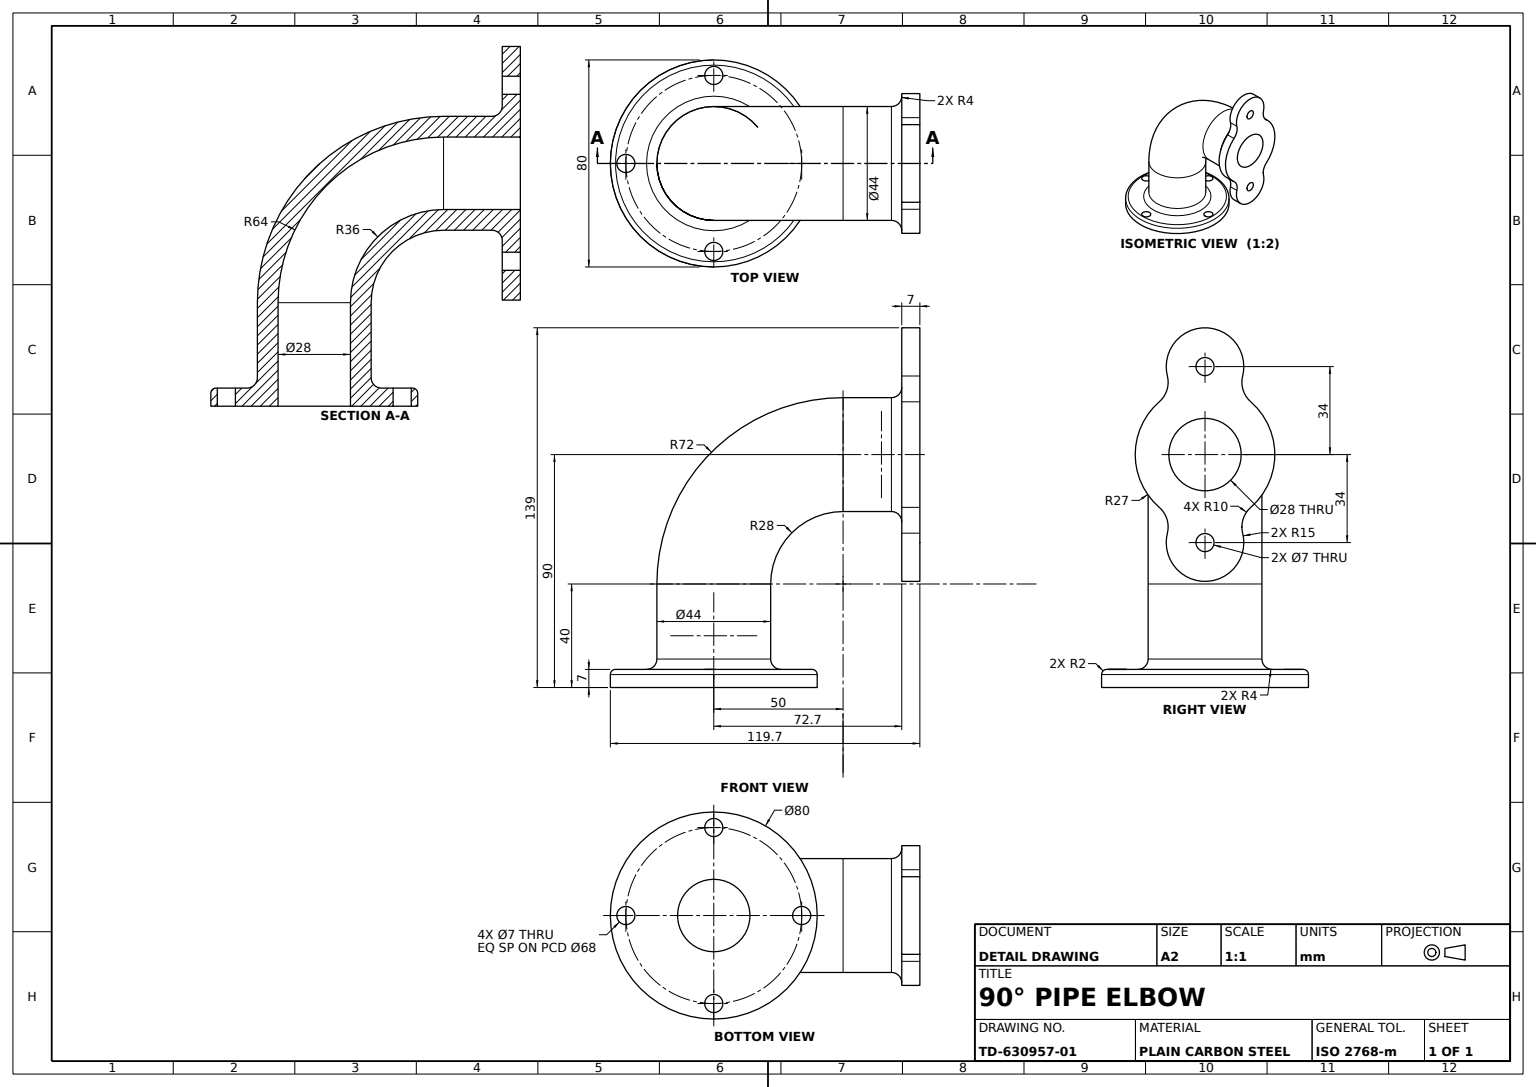
from build123d import *

# Parameters (mm, degrees)
OVAL_FLANGE_SKETCH_R               = 14
OVAL_FLANGE_SKETCH_R_2             = 3.5
OVAL_FLANGE_DEPTH                  = 3.5
PIPE_SECTION_SKETCH_44X_28_R       = 22
PIPE_SECTION_SKETCH_44X_28_R_2     = 14
ROUND_START                        = 7
ROUND_FLANGE_SKETCH_R              = 40
ROUND_FLANGE_SKETCH_R_2            = 14
ROUND_FLANGE_80_DEPTH              = 7
PIPE_TO_FLANGE_FILLETS_R4_R        = 4
ROUND_FLANGE_EDGE_FILLET_R2_R      = 2
ROUND_FLANGE_BOLT_HOLES_SKETCH_R   = 3.5
ROUND_FLANGE_BOLT_HOLES_4X_7_DEPTH = 10


with BuildPart() as part:
    # Oval Flange Sketch → Oval Flange (new, symmetric)
    with BuildSketch(Plane(origin=(0, 0, 0), x_dir=(0, 0, -1), z_dir=(1, 0, 0))):
        with BuildLine():
            ThreePointArc((17.699378464, -20.389507154), (27, 0), (17.699378464, 20.389507154))
            ThreePointArc((17.699378464, 20.389507154), (14.717914983, 24.932911413), (14.552822293, 30.364705882))
            ThreePointArc((14.552822293, 30.364705882), (0, 49), (-14.552822293, 30.364705882))
            ThreePointArc((-14.552822293, 30.364705882), (-14.717914983, 24.932911413), (-17.699378464, 20.389507154))
            ThreePointArc((-17.699378464, 20.389507154), (-27, 0), (-17.699378464, -20.389507154))
            ThreePointArc((-17.699378464, -20.389507154), (-14.717914983, -24.932911413), (-14.552822293, -30.364705882))
            ThreePointArc((-14.552822293, -30.364705882), (0, -49), (14.552822293, -30.364705882))
            ThreePointArc((14.552822293, -30.364705882), (14.717914983, -24.932911413), (17.699378464, -20.389507154))
        make_face()
        Circle(OVAL_FLANGE_SKETCH_R, mode=Mode.SUBTRACT)
        with Locations((0, 34)):
            Circle(OVAL_FLANGE_SKETCH_R_2, mode=Mode.SUBTRACT)
        with Locations((0, -34)):
            Circle(OVAL_FLANGE_SKETCH_R_2, mode=Mode.SUBTRACT)
    extrude(amount=OVAL_FLANGE_DEPTH, both=True)

    # Pipe Elbow Sweep: sweep along a path in Elbow Path Sketch
    with BuildLine(Plane.XY) as pipe_elbow_sweep_path:
        Line((0, 0), (-26.195643288, 0))
        ThreePointArc((-26.195643288, 0), (-61.550982347, -14.644660941), (-76.195643288, -50))
        Line((-76.195643288, -50), (-76.195643288, -83))
    # Pipe Section Sketch Ø44xØ28 → Pipe Elbow Sweep (sweep)
    with BuildSketch(Plane(origin=(0, -83, 0), x_dir=(1, 0, 0), z_dir=(0, 1, 0))):
        with Locations((-76.195643288, 0)):
            Circle(PIPE_SECTION_SKETCH_44X_28_R)
        with Locations((-76.195643288, 0)):
            Circle(PIPE_SECTION_SKETCH_44X_28_R_2, mode=Mode.SUBTRACT)
    sweep(path=pipe_elbow_sweep_path.line)

    # Round Flange Sketch → Round Flange Ø80 (add)
    with BuildSketch(Plane.XZ.offset(83).offset(ROUND_START)):
        with Locations(Location((-76.195643288, 0, 0), (0, 0, 270))):
            Circle(ROUND_FLANGE_SKETCH_R)
        with Locations(Location((-76.195643288, 0, 0), (0, 0, 270))):
            Circle(ROUND_FLANGE_SKETCH_R_2, mode=Mode.SUBTRACT)
    extrude(amount=-ROUND_FLANGE_80_DEPTH)

    # Pipe to Flange Fillets R4
    pipe_to_flange_fillets_r4_edges = [part.edges().sort_by_distance(p)[0] for p in [
        (-3.5, 22, 0),
        (-98.195643288, -83, 0),
    ]]
    fillet(pipe_to_flange_fillets_r4_edges, radius=PIPE_TO_FLANGE_FILLETS_R4_R)

    # Round Flange Edge Fillet R2
    round_flange_edge_fillet_r2_edges = [part.edges().sort_by_distance(p)[0] for p in [
        (-76.195643288, -83, 40),
    ]]
    fillet(round_flange_edge_fillet_r2_edges, radius=ROUND_FLANGE_EDGE_FILLET_R2_R)

    # Round Flange Bolt Holes Sketch → Round Flange Bolt Holes 4xØ7 (cut)
    with BuildSketch(Plane.XZ.offset(90)):
        with Locations(Location((-110.195643288, 0, 0), (0, 0, 270))):
            Circle(ROUND_FLANGE_BOLT_HOLES_SKETCH_R)
        with Locations(Location((-42.195643288, 0, 0), (0, 0, 270))):
            Circle(ROUND_FLANGE_BOLT_HOLES_SKETCH_R)
        with Locations(Location((-76.195643288, 34, 0), (0, 0, 270))):
            Circle(ROUND_FLANGE_BOLT_HOLES_SKETCH_R)
        with Locations(Location((-76.195643288, -34, 0), (0, 0, 270))):
            Circle(ROUND_FLANGE_BOLT_HOLES_SKETCH_R)
    extrude(amount=-ROUND_FLANGE_BOLT_HOLES_4X_7_DEPTH, mode=Mode.SUBTRACT)


solid = part.part
